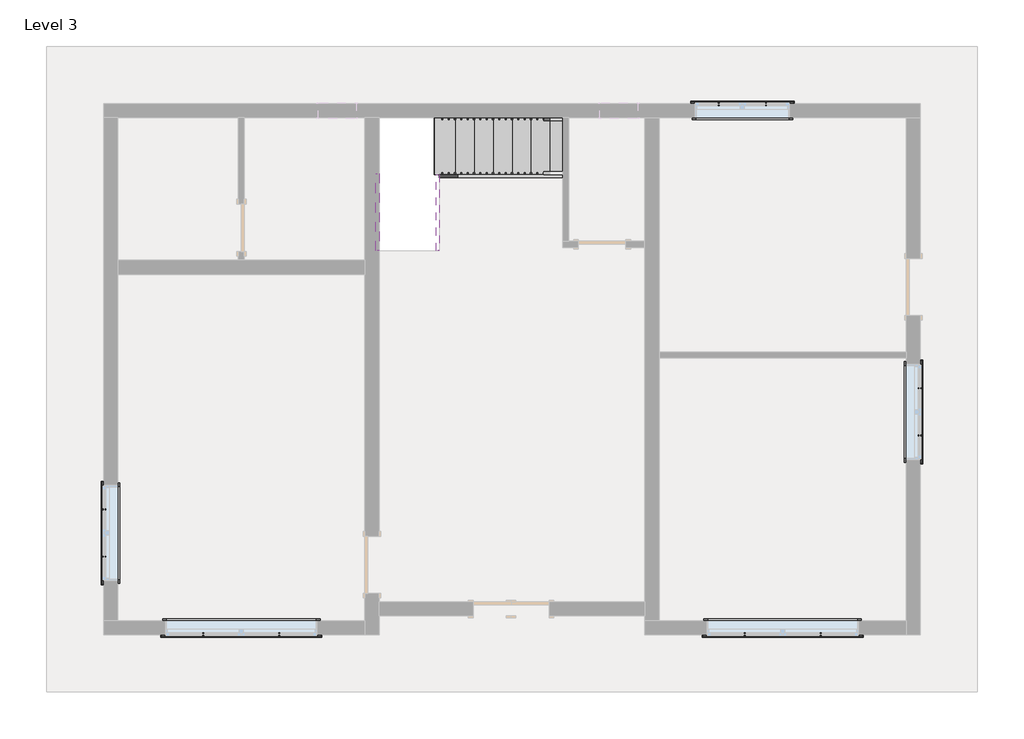
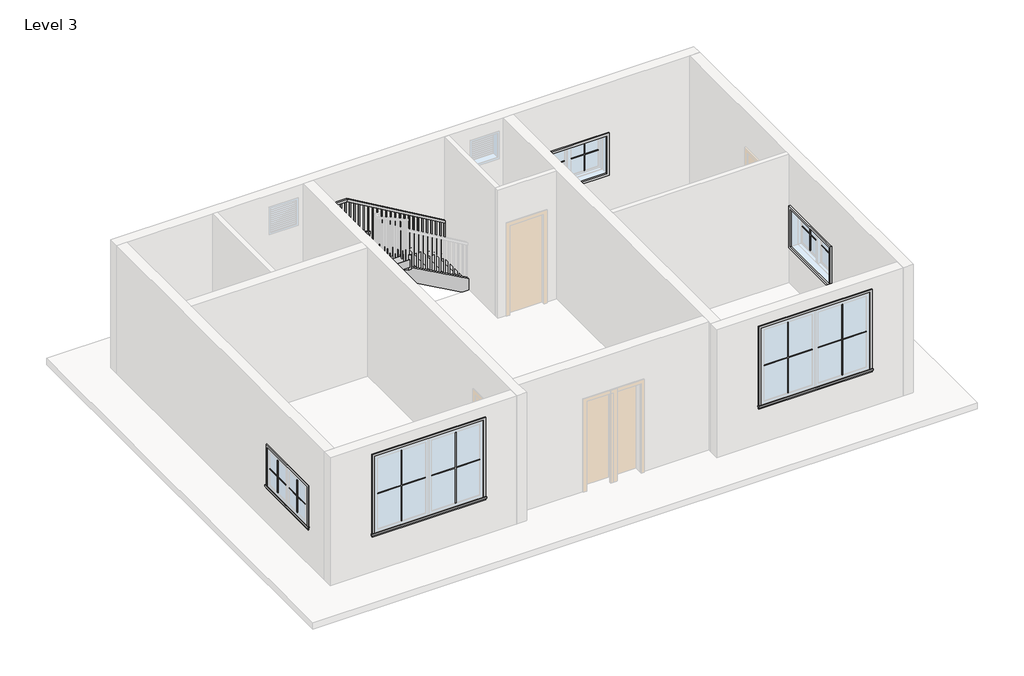
# One storey, part 2 of 2: 20 proxies, 4 members, 1 railing, 1 stair flight.
"""IFC4 building model written with IfcOpenShell, lengths in millimetres."""

from ifc_helpers import new_model, si_unit, frame, origin, place, context, project, spatial, polyline, outline, extrude, faceted_brep, transform, mapped, element, save
from components import muntin_pattern_2x2_muntin_pattern_2x2_9352d081, muntin_pattern_2x2_muntin_pattern_2x2_5c2cbe28, muntin_pattern_2x2_muntin_pattern_2x2_bb8d4d84, muntin_pattern_2x2_muntin_pattern_2x2_d03a1f3c, trim_window_exterior_flat_with_sill_979bde60, trim_window_exterior_flat_with_sill_359ed2ce, trim_window_interior_flat_picture_frame_7883d11b, trim_window_interior_flat_picture_frame_939a8053, stair_flight_1226b75b

model = new_model("IFC4")

# Units and contexts
model_context = context("Model", 3, world=origin())
ifc_project = project(units=[si_unit("LENGTHUNIT", "METRE", prefix="MILLI")], contexts=[model_context])

# Site, building, storey
site = spatial("IfcSite", under=ifc_project)
building = spatial("IfcBuilding", under=site)
storey = spatial("IfcBuildingStorey", under=building, Name="Level 3", Elevation=6248.4)

# Proxies
placement = place(None, origin())
muntin_pattern_2x2_muntin_pattern_2x2_shape = muntin_pattern_2x2_muntin_pattern_2x2_9352d081(model_context)
element("IfcBuildingElementProxy", 1, Name="Muntin Pattern_2x2 : Muntin Pattern_2x2", ObjectType="Muntin Pattern_2x2 : Muntin Pattern_2x2", at=placement, inside=storey, context=model_context, shape_type="MappedRepresentation", body=[
    mapped(muntin_pattern_2x2_muntin_pattern_2x2_shape, transform((-7798.9165084, -1764.5743005, 7232.65), x_axis=(0.0, 1.0, 0.0), y_axis=(-1.0, 0.0, 0.0), z_axis=(0.0, 0.0, 1.0))),
])
element("IfcBuildingElementProxy", 2, Name="Muntin Pattern_2x2 : Muntin Pattern_2x2", ObjectType="Muntin Pattern_2x2 : Muntin Pattern_2x2", at=placement, inside=storey, context=model_context, shape_type="MappedRepresentation", body=[
    mapped(muntin_pattern_2x2_muntin_pattern_2x2_shape, transform((5288.4334916, 937.3506995, 7232.65), x_axis=(0.0, -1.0, 0.0), y_axis=(1.0, 0.0, 0.0), z_axis=(0.0, 0.0, 1.0))),
])
element("IfcBuildingElementProxy", 3, Name="Muntin Pattern_2x2 : Muntin Pattern_2x2", ObjectType="Muntin Pattern_2x2 : Muntin Pattern_2x2", at=placement, inside=storey, context=model_context, shape_type="MappedRepresentation", body=[
    mapped(muntin_pattern_2x2_muntin_pattern_2x2_shape, transform((2061.0459916, 5501.4131995, 7232.65), x_axis=(1.0, 0.0, 0.0), y_axis=(0.0, 1.0, 0.0), z_axis=(0.0, 0.0, 1.0))),
])
muntin_pattern_2x2_muntin_pattern_2x2_2_shape = muntin_pattern_2x2_muntin_pattern_2x2_5c2cbe28(model_context)
element("IfcBuildingElementProxy", 4, Name="Muntin Pattern_2x2 : Muntin Pattern_2x2", ObjectType="Muntin Pattern_2x2 : Muntin Pattern_2x2", at=placement, inside=storey, context=model_context, shape_type="MappedRepresentation", body=[
    mapped(muntin_pattern_2x2_muntin_pattern_2x2_2_shape, transform((-7798.9165084, -1005.7493005, 7232.65), x_axis=(0.0, -1.0, 0.0), y_axis=(1.0, 0.0, 0.0), z_axis=(0.0, 0.0, 1.0))),
])
element("IfcBuildingElementProxy", 5, Name="Muntin Pattern_2x2 : Muntin Pattern_2x2", ObjectType="Muntin Pattern_2x2 : Muntin Pattern_2x2", at=placement, inside=storey, context=model_context, shape_type="MappedRepresentation", body=[
    mapped(muntin_pattern_2x2_muntin_pattern_2x2_2_shape, transform((5288.4334916, 178.5256995, 7232.65), x_axis=(0.0, 1.0, 0.0), y_axis=(-1.0, 0.0, 0.0), z_axis=(0.0, 0.0, 1.0))),
])
element("IfcBuildingElementProxy", 6, Name="Muntin Pattern_2x2 : Muntin Pattern_2x2", ObjectType="Muntin Pattern_2x2 : Muntin Pattern_2x2", at=placement, inside=storey, context=model_context, shape_type="MappedRepresentation", body=[
    mapped(muntin_pattern_2x2_muntin_pattern_2x2_2_shape, transform((2819.8709916, 5501.4131995, 7232.65), x_axis=(-1.0, 0.0, 0.0), y_axis=(0.0, -1.0, 0.0), z_axis=(0.0, 0.0, 1.0))),
])
muntin_pattern_2x2_muntin_pattern_2x2_3_shape = muntin_pattern_2x2_muntin_pattern_2x2_bb8d4d84(model_context)
element("IfcBuildingElementProxy", 7, Name="Muntin Pattern_2x2 : Muntin Pattern_2x2", ObjectType="Muntin Pattern_2x2 : Muntin Pattern_2x2", at=placement, inside=storey, context=model_context, shape_type="MappedRepresentation", body=[
    mapped(muntin_pattern_2x2_muntin_pattern_2x2_3_shape, transform((-4990.6290084, -3013.9368005, 7232.65), x_axis=(-1.0, 0.0, 0.0), y_axis=(0.0, -1.0, 0.0), z_axis=(0.0, 0.0, 1.0))),
])
element("IfcBuildingElementProxy", 8, Name="Muntin Pattern_2x2 : Muntin Pattern_2x2", ObjectType="Muntin Pattern_2x2 : Muntin Pattern_2x2", at=placement, inside=storey, context=model_context, shape_type="MappedRepresentation", body=[
    mapped(muntin_pattern_2x2_muntin_pattern_2x2_3_shape, transform((3696.1709916, -3013.9368005, 7232.65), x_axis=(-1.0, 0.0, 0.0), y_axis=(0.0, -1.0, 0.0), z_axis=(0.0, 0.0, 1.0))),
])
muntin_pattern_2x2_muntin_pattern_2x2_4_shape = muntin_pattern_2x2_muntin_pattern_2x2_d03a1f3c(model_context)
element("IfcBuildingElementProxy", 9, Name="Muntin Pattern_2x2 : Muntin Pattern_2x2", ObjectType="Muntin Pattern_2x2 : Muntin Pattern_2x2", at=placement, inside=storey, context=model_context, shape_type="MappedRepresentation", body=[
    mapped(muntin_pattern_2x2_muntin_pattern_2x2_4_shape, transform((-6206.6540084, -3013.9368005, 7232.65), x_axis=(1.0, 0.0, 0.0), y_axis=(0.0, 1.0, 0.0), z_axis=(0.0, 0.0, 1.0))),
])
element("IfcBuildingElementProxy", 10, Name="Muntin Pattern_2x2 : Muntin Pattern_2x2", ObjectType="Muntin Pattern_2x2 : Muntin Pattern_2x2", at=placement, inside=storey, context=model_context, shape_type="MappedRepresentation", body=[
    mapped(muntin_pattern_2x2_muntin_pattern_2x2_4_shape, transform((2480.1459916, -3013.9368005, 7232.65), x_axis=(1.0, 0.0, 0.0), y_axis=(0.0, 1.0, 0.0), z_axis=(0.0, 0.0, 1.0))),
])
trim_window_exterior_flat_with_sill_shape = trim_window_exterior_flat_with_sill_979bde60(model_context)
element("IfcBuildingElementProxy", 11, Name="Trim-Window-Exterior-Flat : with Sill", ObjectType="Trim-Window-Exterior-Flat : with Sill", at=placement, inside=storey, context=model_context, shape_type="MappedRepresentation", body=[
    mapped(trim_window_exterior_flat_with_sill_shape, transform((-7808.4415084, -1385.1618005, 8077.2), x_axis=(0.0, -1.0, 0.0), y_axis=(0.0, 0.0, 1.0), z_axis=(-1.0, 0.0, 0.0))),
])
element("IfcBuildingElementProxy", 12, Name="Trim-Window-Exterior-Flat : with Sill", ObjectType="Trim-Window-Exterior-Flat : with Sill", at=placement, inside=storey, context=model_context, shape_type="MappedRepresentation", body=[
    mapped(trim_window_exterior_flat_with_sill_shape, transform((5297.9584916, 557.9381995, 8077.2), x_axis=(0.0, 1.0, 0.0), y_axis=(0.0, 0.0, 1.0), z_axis=(1.0, 0.0, 0.0))),
])
element("IfcBuildingElementProxy", 13, Name="Trim-Window-Exterior-Flat : with Sill", ObjectType="Trim-Window-Exterior-Flat : with Sill", at=placement, inside=storey, context=model_context, shape_type="MappedRepresentation", body=[
    mapped(trim_window_exterior_flat_with_sill_shape, transform((2440.4584916, 5510.9381995, 8077.2), x_axis=(-1.0, 0.0, 0.0), y_axis=(0.0, 0.0, 1.0), z_axis=(0.0, 1.0, 0.0))),
])
trim_window_exterior_flat_with_sill_2_shape = trim_window_exterior_flat_with_sill_359ed2ce(model_context)
element("IfcBuildingElementProxy", 14, Name="Trim-Window-Exterior-Flat : with Sill", ObjectType="Trim-Window-Exterior-Flat : with Sill", at=placement, inside=storey, context=model_context, shape_type="MappedRepresentation", body=[
    mapped(trim_window_exterior_flat_with_sill_2_shape, transform((-5598.6415084, -3023.4618005, 8991.6), x_axis=(1.0, 0.0, 0.0), y_axis=(0.0, 0.0, 1.0), z_axis=(0.0, -1.0, 0.0))),
])
element("IfcBuildingElementProxy", 15, Name="Trim-Window-Exterior-Flat : with Sill", ObjectType="Trim-Window-Exterior-Flat : with Sill", at=placement, inside=storey, context=model_context, shape_type="MappedRepresentation", body=[
    mapped(trim_window_exterior_flat_with_sill_2_shape, transform((3088.1584916, -3023.4618005, 8991.6), x_axis=(1.0, 0.0, 0.0), y_axis=(0.0, 0.0, 1.0), z_axis=(0.0, -1.0, 0.0))),
])
trim_window_interior_flat_picture_frame_shape = trim_window_interior_flat_picture_frame_7883d11b(model_context)
element("IfcBuildingElementProxy", 16, Name="Trim-Window-Interior-Flat : Picture Frame", ObjectType="Trim-Window-Interior-Flat : Picture Frame", at=placement, inside=storey, context=model_context, shape_type="MappedRepresentation", body=[
    mapped(trim_window_interior_flat_picture_frame_shape, transform((-7579.8415084, -1385.1618005, 8077.2), x_axis=(0.0, 1.0, 0.0), y_axis=(0.0, 0.0, 1.0), z_axis=(1.0, 0.0, 0.0))),
])
element("IfcBuildingElementProxy", 17, Name="Trim-Window-Interior-Flat : Picture Frame", ObjectType="Trim-Window-Interior-Flat : Picture Frame", at=placement, inside=storey, context=model_context, shape_type="MappedRepresentation", body=[
    mapped(trim_window_interior_flat_picture_frame_shape, transform((5069.3584916, 557.9381995, 8077.2), x_axis=(0.0, -1.0, 0.0), y_axis=(0.0, 0.0, 1.0), z_axis=(-1.0, 0.0, 0.0))),
])
element("IfcBuildingElementProxy", 18, Name="Trim-Window-Interior-Flat : Picture Frame", ObjectType="Trim-Window-Interior-Flat : Picture Frame", at=placement, inside=storey, context=model_context, shape_type="MappedRepresentation", body=[
    mapped(trim_window_interior_flat_picture_frame_shape, transform((2440.4584916, 5282.3381995, 8077.2), x_axis=(1.0, 0.0, 0.0), y_axis=(0.0, 0.0, 1.0), z_axis=(0.0, -1.0, 0.0))),
])
trim_window_interior_flat_picture_frame_2_shape = trim_window_interior_flat_picture_frame_939a8053(model_context)
element("IfcBuildingElementProxy", 19, Name="Trim-Window-Interior-Flat : Picture Frame", ObjectType="Trim-Window-Interior-Flat : Picture Frame", at=placement, inside=storey, context=model_context, shape_type="MappedRepresentation", body=[
    mapped(trim_window_interior_flat_picture_frame_2_shape, transform((-5598.6415084, -2794.8618005, 8991.6), x_axis=(-1.0, 0.0, 0.0), y_axis=(0.0, 0.0, 1.0), z_axis=(0.0, 1.0, 0.0))),
])
element("IfcBuildingElementProxy", 20, Name="Trim-Window-Interior-Flat : Picture Frame", ObjectType="Trim-Window-Interior-Flat : Picture Frame", at=placement, inside=storey, context=model_context, shape_type="MappedRepresentation", body=[
    mapped(trim_window_interior_flat_picture_frame_2_shape, transform((3088.1584916, -2794.8618005, 8991.6), x_axis=(-1.0, 0.0, 0.0), y_axis=(0.0, 0.0, 1.0), z_axis=(0.0, 1.0, 0.0))),
])

# Members
element("IfcMember", 21, ObjectType="Stringer - 2\" Width", at=placement, inside=storey, context=model_context, shape_type="SweptSolid", body=[
    extrude(outline(polyline([(6248.4, -442.4415084), (6512.4428392, -442.4415084), (7613.1095059, -2423.6415084), (7264.4308318, -2423.6415084), (6248.4, -594.7860112), (6248.4, -442.4415084)])), frame((0.0, 4317.5146777, 0.0), z_axis=(0.0, 1.0, 0.0), x_axis=(0.0, 0.0, 1.0)), (0.0, 0.0, 1.0), 50.8),
])
element("IfcMember", 22, ObjectType="Stringer - 2\" Width", at=placement, inside=storey, context=model_context, shape_type="SweptSolid", body=[
    extrude(outline(polyline([(4368.3146777, 7810.645537), (4368.3146777, 7462.0006925), (3148.7383287, 8139.2643411), (3148.7383287, 8487.9091856), (4368.3146777, 7810.645537)])), frame((-2474.4415084, 0.0, 0.0), z_axis=(1.0, 0.0, 0.0), x_axis=(0.0, 1.0, 0.0)), (0.0, 0.0, 1.0), 50.8),
])
element("IfcMember", 23, ObjectType="Stringer - 2\" Width", at=placement, inside=storey, context=model_context, shape_type="SweptSolid", body=[
    extrude(outline(polyline([(6248.4, -442.4415084), (6512.4428392, -442.4415084), (7303.0636166, -1865.5589077), (7303.0636166, -2493.1805211), (6248.4, -594.7860112), (6248.4, -442.4415084)])), frame((0.0, 5282.3381995, 0.0), z_axis=(0.0, 1.0, 0.0), x_axis=(0.0, 0.0, 1.0)), (0.0, 0.0, 1.0), 50.8),
])
element("IfcMember", 24, ObjectType="Stringer - 2\" Width", at=placement, inside=storey, context=model_context, shape_type="SweptSolid", body=[
    extrude(outline(polyline([(3758.489521, 7800.653054), (3148.7383287, 8139.2643411), (3148.7383287, 8487.9091856), (4386.3085505, 7800.653054), (3758.489521, 7800.653054)])), frame((-3439.6415084, 0.0, 0.0), z_axis=(1.0, 0.0, 0.0), x_axis=(0.0, 1.0, 0.0)), (0.0, 0.0, 1.0), 50.8),
])

# Railing
element("IfcRailing", 25, ObjectType="Handrail - Rectangular", at=placement, inside=storey, context=model_context, shape_type="SolidModel", body=[
    faceted_brep([(-442.4415084, 5231.5381995, 7332.1333333), (-442.4415084, 5231.5381995, 7273.3219871), (-442.4415084, 5282.3381995, 7273.3219871), (-442.4415084, 5282.3381995, 7332.1333333), (-2641.0608886, 5231.5381995, 8614.6613051), (-2654.794625, 5231.5381995, 8563.8613051), (-2654.794625, 5282.3381995, 8563.8613051), (-2641.0608886, 5282.3381995, 8614.6613051), (-3338.0415084, 5231.5381995, 8614.6613051), (-3338.0415084, 5231.5381995, 8563.8613051), (-3388.8415084, 5282.3381995, 8563.8613051), (-3388.8415084, 5282.3381995, 8614.6613051), (-3338.0415084, 4498.2044111, 8614.6613051), (-3338.0415084, 4485.04436, 8563.8613051), (-3388.8415084, 4485.04436, 8563.8613051), (-3388.8415084, 4498.2044111, 8614.6613051), (-3338.0415084, 3148.7383287, 9364.1333333), (-3388.8415084, 3148.7383287, 9364.1333333), (-3388.8415084, 3148.7383287, 9306.02445), (-3338.0415084, 3148.7383287, 9306.02445)], [[[0, 1, 2, 3]], [[1, 0, 4, 5]], [[2, 1, 5, 6]], [[3, 2, 6, 7]], [[0, 3, 7, 4]], [[5, 4, 8, 9]], [[6, 5, 9, 10]], [[7, 6, 10, 11]], [[4, 7, 11, 8]], [[9, 8, 12, 13]], [[10, 9, 13, 14]], [[11, 10, 14, 15]], [[8, 11, 15, 12]], [[16, 17, 18, 19]], [[13, 12, 16, 19]], [[14, 13, 19, 18]], [[15, 14, 18, 17]], [[12, 15, 17, 16]]]),
    extrude(outline(polyline([(3215.4131995, 9268.9942858), (3234.4631995, 9258.4142183), (3234.4631995, 8280.4), (3215.4131995, 8280.4), (3215.4131995, 9268.9942858)])), frame((-3372.9665084, 0.0, 0.0), z_axis=(1.0, 0.0, 0.0), x_axis=(0.0, 1.0, 0.0)), (0.0, 0.0, 1.0), 19.05),
    extrude(outline(polyline([(3317.0131995, 9212.7240232), (3336.0631995, 9202.1439558), (3336.0631995, 8280.4), (3317.0131995, 8280.4), (3317.0131995, 9212.7240232)])), frame((-3372.9665084, 0.0, 0.0), z_axis=(1.0, 0.0, 0.0), x_axis=(0.0, 1.0, 0.0)), (0.0, 0.0, 1.0), 19.05),
    extrude(outline(polyline([(3418.6131995, 9156.2969969), (3437.6631995, 9145.7169295), (3437.6631995, 8280.4), (3418.6131995, 8280.4), (3418.6131995, 9156.2969969)])), frame((-3372.9665084, 0.0, 0.0), z_axis=(1.0, 0.0, 0.0), x_axis=(0.0, 1.0, 0.0)), (0.0, 0.0, 1.0), 19.05),
    extrude(outline(polyline([(3520.2131995, 9099.8699707), (3539.2631995, 9089.2899033), (3539.2631995, 8111.0666667), (3520.2131995, 8111.0666667), (3520.2131995, 9099.8699707)])), frame((-3372.9665084, 0.0, 0.0), z_axis=(1.0, 0.0, 0.0), x_axis=(0.0, 1.0, 0.0)), (0.0, 0.0, 1.0), 19.05),
    extrude(outline(polyline([(3621.8131995, 9043.3906899), (3640.8631995, 9032.8106224), (3640.8631995, 8111.0666667), (3621.8131995, 8111.0666667), (3621.8131995, 9043.3906899)])), frame((-3372.9665084, 0.0, 0.0), z_axis=(1.0, 0.0, 0.0), x_axis=(0.0, 1.0, 0.0)), (0.0, 0.0, 1.0), 19.05),
    extrude(outline(polyline([(3723.4131995, 8986.9636636), (3742.4631995, 8976.3835962), (3742.4631995, 8111.0666667), (3723.4131995, 8111.0666667), (3723.4131995, 8986.9636636)])), frame((-3372.9665084, 0.0, 0.0), z_axis=(1.0, 0.0, 0.0), x_axis=(0.0, 1.0, 0.0)), (0.0, 0.0, 1.0), 19.05),
    extrude(outline(polyline([(3825.0131995, 8930.5366374), (3844.0631995, 8919.9565699), (3844.0631995, 7941.7333333), (3825.0131995, 7941.7333333), (3825.0131995, 8930.5366374)])), frame((-3372.9665084, 0.0, 0.0), z_axis=(1.0, 0.0, 0.0), x_axis=(0.0, 1.0, 0.0)), (0.0, 0.0, 1.0), 19.05),
    extrude(outline(polyline([(3926.6131995, 8874.0573565), (3945.6631995, 8863.4772891), (3945.6631995, 7941.7333333), (3926.6131995, 7941.7333333), (3926.6131995, 8874.0573565)])), frame((-3372.9665084, 0.0, 0.0), z_axis=(1.0, 0.0, 0.0), x_axis=(0.0, 1.0, 0.0)), (0.0, 0.0, 1.0), 19.05),
    extrude(outline(polyline([(4028.2131995, 8817.6303303), (4047.2631995, 8807.0502629), (4047.2631995, 7941.7333333), (4028.2131995, 7941.7333333), (4028.2131995, 8817.6303303)])), frame((-3372.9665084, 0.0, 0.0), z_axis=(1.0, 0.0, 0.0), x_axis=(0.0, 1.0, 0.0)), (0.0, 0.0, 1.0), 19.05),
    extrude(outline(polyline([(4129.8131995, 8761.203304), (4148.8631995, 8750.6232366), (4148.8631995, 7772.4), (4129.8131995, 7772.4), (4129.8131995, 8761.203304)])), frame((-3372.9665084, 0.0, 0.0), z_axis=(1.0, 0.0, 0.0), x_axis=(0.0, 1.0, 0.0)), (0.0, 0.0, 1.0), 19.05),
    extrude(outline(polyline([(4231.4131995, 8704.7240232), (4250.4631995, 8694.1439558), (4250.4631995, 7772.4), (4231.4131995, 7772.4), (4231.4131995, 8704.7240232)])), frame((-3372.9665084, 0.0, 0.0), z_axis=(1.0, 0.0, 0.0), x_axis=(0.0, 1.0, 0.0)), (0.0, 0.0, 1.0), 19.05),
    extrude(outline(polyline([(4333.0131995, 8648.2969969), (4352.0631995, 8637.7169295), (4352.0631995, 7772.4), (4333.0131995, 7772.4), (4333.0131995, 8648.2969969)])), frame((-3372.9665084, 0.0, 0.0), z_axis=(1.0, 0.0, 0.0), x_axis=(0.0, 1.0, 0.0)), (0.0, 0.0, 1.0), 19.05),
    extrude(outline(polyline([(4434.6131995, 8591.8699707), (4453.6631995, 8581.2899033), (4453.6631995, 7603.0666667), (4434.6131995, 7603.0666667), (4434.6131995, 8591.8699707)])), frame((-3372.9665084, 0.0, 0.0), z_axis=(1.0, 0.0, 0.0), x_axis=(0.0, 1.0, 0.0)), (0.0, 0.0, 1.0), 19.05),
    extrude(outline(polyline([(-3372.9665084, 4555.2631995), (-3353.9165084, 4555.2631995), (-3353.9165084, 4536.2131995), (-3372.9665084, 4536.2131995), (-3372.9665084, 4555.2631995)])), frame((0.0, 0.0, 7603.0666667), z_axis=(0.0, 0.0, 1.0), x_axis=(1.0, 0.0, 0.0)), (0.0, 0.0, 1.0), 960.7946385),
    extrude(outline(polyline([(-3372.9665084, 4656.8631995), (-3353.9165084, 4656.8631995), (-3353.9165084, 4637.8131995), (-3372.9665084, 4637.8131995), (-3372.9665084, 4656.8631995)])), frame((0.0, 0.0, 7603.0666667), z_axis=(0.0, 0.0, 1.0), x_axis=(1.0, 0.0, 0.0)), (0.0, 0.0, 1.0), 960.7946385),
    extrude(outline(polyline([(-3372.9665084, 4758.4631995), (-3353.9165084, 4758.4631995), (-3353.9165084, 4739.4131995), (-3372.9665084, 4739.4131995), (-3372.9665084, 4758.4631995)])), frame((0.0, 0.0, 7603.0666667), z_axis=(0.0, 0.0, 1.0), x_axis=(1.0, 0.0, 0.0)), (0.0, 0.0, 1.0), 960.7946385),
    extrude(outline(polyline([(-3372.9665084, 4860.0631995), (-3353.9165084, 4860.0631995), (-3353.9165084, 4841.0131995), (-3372.9665084, 4841.0131995), (-3372.9665084, 4860.0631995)])), frame((0.0, 0.0, 7603.0666667), z_axis=(0.0, 0.0, 1.0), x_axis=(1.0, 0.0, 0.0)), (0.0, 0.0, 1.0), 960.7946385),
    extrude(outline(polyline([(-3372.9665084, 4961.6631995), (-3353.9165084, 4961.6631995), (-3353.9165084, 4942.6131995), (-3372.9665084, 4942.6131995), (-3372.9665084, 4961.6631995)])), frame((0.0, 0.0, 7603.0666667), z_axis=(0.0, 0.0, 1.0), x_axis=(1.0, 0.0, 0.0)), (0.0, 0.0, 1.0), 960.7946385),
    extrude(outline(polyline([(-3372.9665084, 5063.2631995), (-3353.9165084, 5063.2631995), (-3353.9165084, 5044.2131995), (-3372.9665084, 5044.2131995), (-3372.9665084, 5063.2631995)])), frame((0.0, 0.0, 7603.0666667), z_axis=(0.0, 0.0, 1.0), x_axis=(1.0, 0.0, 0.0)), (0.0, 0.0, 1.0), 960.7946385),
    extrude(outline(polyline([(-3372.9665084, 5164.8631995), (-3353.9165084, 5164.8631995), (-3353.9165084, 5145.8131995), (-3372.9665084, 5145.8131995), (-3372.9665084, 5164.8631995)])), frame((0.0, 0.0, 7603.0666667), z_axis=(0.0, 0.0, 1.0), x_axis=(1.0, 0.0, 0.0)), (0.0, 0.0, 1.0), 960.7946385),
    extrude(outline(polyline([(-3277.7165084, 5266.4631995), (-3277.7165084, 5247.4131995), (-3296.7665084, 5247.4131995), (-3296.7665084, 5266.4631995), (-3277.7165084, 5266.4631995)])), frame((0.0, 0.0, 7603.0666667), z_axis=(0.0, 0.0, 1.0), x_axis=(1.0, 0.0, 0.0)), (0.0, 0.0, 1.0), 960.7946385),
    extrude(outline(polyline([(-3176.1165084, 5266.4631995), (-3176.1165084, 5247.4131995), (-3195.1665084, 5247.4131995), (-3195.1665084, 5266.4631995), (-3176.1165084, 5266.4631995)])), frame((0.0, 0.0, 7603.0666667), z_axis=(0.0, 0.0, 1.0), x_axis=(1.0, 0.0, 0.0)), (0.0, 0.0, 1.0), 960.7946385),
    extrude(outline(polyline([(-3074.5165084, 5266.4631995), (-3074.5165084, 5247.4131995), (-3093.5665084, 5247.4131995), (-3093.5665084, 5266.4631995), (-3074.5165084, 5266.4631995)])), frame((0.0, 0.0, 7603.0666667), z_axis=(0.0, 0.0, 1.0), x_axis=(1.0, 0.0, 0.0)), (0.0, 0.0, 1.0), 960.7946385),
    extrude(outline(polyline([(-2972.9165084, 5266.4631995), (-2972.9165084, 5247.4131995), (-2991.9665084, 5247.4131995), (-2991.9665084, 5266.4631995), (-2972.9165084, 5266.4631995)])), frame((0.0, 0.0, 7603.0666667), z_axis=(0.0, 0.0, 1.0), x_axis=(1.0, 0.0, 0.0)), (0.0, 0.0, 1.0), 960.7946385),
    extrude(outline(polyline([(-2871.3165084, 5266.4631995), (-2871.3165084, 5247.4131995), (-2890.3665084, 5247.4131995), (-2890.3665084, 5266.4631995), (-2871.3165084, 5266.4631995)])), frame((0.0, 0.0, 7603.0666667), z_axis=(0.0, 0.0, 1.0), x_axis=(1.0, 0.0, 0.0)), (0.0, 0.0, 1.0), 960.7946385),
    extrude(outline(polyline([(-2769.7165084, 5266.4631995), (-2769.7165084, 5247.4131995), (-2788.7665084, 5247.4131995), (-2788.7665084, 5266.4631995), (-2769.7165084, 5266.4631995)])), frame((0.0, 0.0, 7603.0666667), z_axis=(0.0, 0.0, 1.0), x_axis=(1.0, 0.0, 0.0)), (0.0, 0.0, 1.0), 960.7946385),
    extrude(outline(polyline([(-2668.1165084, 5266.4631995), (-2668.1165084, 5247.4131995), (-2687.1665084, 5247.4131995), (-2687.1665084, 5266.4631995), (-2668.1165084, 5266.4631995)])), frame((0.0, 0.0, 7603.0666667), z_axis=(0.0, 0.0, 1.0), x_axis=(1.0, 0.0, 0.0)), (0.0, 0.0, 1.0), 960.7946385),
    extrude(outline(polyline([(8512.3657371, -2566.5165084), (8523.4782371, -2585.5665084), (7603.0666667, -2585.5665084), (7603.0666667, -2566.5165084), (8512.3657371, -2566.5165084)])), frame((0.0, 5247.4131995, 0.0), z_axis=(0.0, 1.0, 0.0), x_axis=(0.0, 0.0, 1.0)), (0.0, 0.0, 1.0), 19.05),
    extrude(outline(polyline([(8453.0990704, -2464.9165084), (8464.2115704, -2483.9665084), (7603.0666667, -2483.9665084), (7603.0666667, -2464.9165084), (8453.0990704, -2464.9165084)])), frame((0.0, 5247.4131995, 0.0), z_axis=(0.0, 1.0, 0.0), x_axis=(0.0, 0.0, 1.0)), (0.0, 0.0, 1.0), 19.05),
    extrude(outline(polyline([(8393.8324038, -2363.3165084), (8404.9449038, -2382.3665084), (7433.7333333, -2382.3665084), (7433.7333333, -2363.3165084), (8393.8324038, -2363.3165084)])), frame((0.0, 5247.4131995, 0.0), z_axis=(0.0, 1.0, 0.0), x_axis=(0.0, 0.0, 1.0)), (0.0, 0.0, 1.0), 19.05),
    extrude(outline(polyline([(8334.5657371, -2261.7165084), (8345.6782371, -2280.7665084), (7433.7333333, -2280.7665084), (7433.7333333, -2261.7165084), (8334.5657371, -2261.7165084)])), frame((0.0, 5247.4131995, 0.0), z_axis=(0.0, 1.0, 0.0), x_axis=(0.0, 0.0, 1.0)), (0.0, 0.0, 1.0), 19.05),
    extrude(outline(polyline([(8275.2990704, -2160.1165084), (8286.4115704, -2179.1665084), (7433.7333333, -2179.1665084), (7433.7333333, -2160.1165084), (8275.2990704, -2160.1165084)])), frame((0.0, 5247.4131995, 0.0), z_axis=(0.0, 1.0, 0.0), x_axis=(0.0, 0.0, 1.0)), (0.0, 0.0, 1.0), 19.05),
    extrude(outline(polyline([(8216.0324038, -2058.5165084), (8227.1449038, -2077.5665084), (7264.4, -2077.5665084), (7264.4, -2058.5165084), (8216.0324038, -2058.5165084)])), frame((0.0, 5247.4131995, 0.0), z_axis=(0.0, 1.0, 0.0), x_axis=(0.0, 0.0, 1.0)), (0.0, 0.0, 1.0), 19.05),
    extrude(outline(polyline([(8156.7657371, -1956.9165084), (8167.8782371, -1975.9665084), (7264.4, -1975.9665084), (7264.4, -1956.9165084), (8156.7657371, -1956.9165084)])), frame((0.0, 5247.4131995, 0.0), z_axis=(0.0, 1.0, 0.0), x_axis=(0.0, 0.0, 1.0)), (0.0, 0.0, 1.0), 19.05),
    extrude(outline(polyline([(8097.4990704, -1855.3165084), (8108.6115704, -1874.3665084), (7264.4, -1874.3665084), (7264.4, -1855.3165084), (8097.4990704, -1855.3165084)])), frame((0.0, 5247.4131995, 0.0), z_axis=(0.0, 1.0, 0.0), x_axis=(0.0, 0.0, 1.0)), (0.0, 0.0, 1.0), 19.05),
    extrude(outline(polyline([(8038.2324038, -1753.7165084), (8049.3449038, -1772.7665084), (7095.0666667, -1772.7665084), (7095.0666667, -1753.7165084), (8038.2324038, -1753.7165084)])), frame((0.0, 5247.4131995, 0.0), z_axis=(0.0, 1.0, 0.0), x_axis=(0.0, 0.0, 1.0)), (0.0, 0.0, 1.0), 19.05),
    extrude(outline(polyline([(7978.9657371, -1652.1165084), (7990.0782371, -1671.1665084), (7095.0666667, -1671.1665084), (7095.0666667, -1652.1165084), (7978.9657371, -1652.1165084)])), frame((0.0, 5247.4131995, 0.0), z_axis=(0.0, 1.0, 0.0), x_axis=(0.0, 0.0, 1.0)), (0.0, 0.0, 1.0), 19.05),
    extrude(outline(polyline([(7919.6990704, -1550.5165084), (7930.8115704, -1569.5665084), (7095.0666667, -1569.5665084), (7095.0666667, -1550.5165084), (7919.6990704, -1550.5165084)])), frame((0.0, 5247.4131995, 0.0), z_axis=(0.0, 1.0, 0.0), x_axis=(0.0, 0.0, 1.0)), (0.0, 0.0, 1.0), 19.05),
    extrude(outline(polyline([(7860.4324038, -1448.9165084), (7871.5449038, -1467.9665084), (6925.7333333, -1467.9665084), (6925.7333333, -1448.9165084), (7860.4324038, -1448.9165084)])), frame((0.0, 5247.4131995, 0.0), z_axis=(0.0, 1.0, 0.0), x_axis=(0.0, 0.0, 1.0)), (0.0, 0.0, 1.0), 19.05),
    extrude(outline(polyline([(7801.1657371, -1347.3165084), (7812.2782371, -1366.3665084), (6925.7333333, -1366.3665084), (6925.7333333, -1347.3165084), (7801.1657371, -1347.3165084)])), frame((0.0, 5247.4131995, 0.0), z_axis=(0.0, 1.0, 0.0), x_axis=(0.0, 0.0, 1.0)), (0.0, 0.0, 1.0), 19.05),
    extrude(outline(polyline([(7741.8990704, -1245.7165084), (7753.0115704, -1264.7665084), (6925.7333333, -1264.7665084), (6925.7333333, -1245.7165084), (7741.8990704, -1245.7165084)])), frame((0.0, 5247.4131995, 0.0), z_axis=(0.0, 1.0, 0.0), x_axis=(0.0, 0.0, 1.0)), (0.0, 0.0, 1.0), 19.05),
    extrude(outline(polyline([(7682.6324038, -1144.1165084), (7693.7449038, -1163.1665084), (6756.4, -1163.1665084), (6756.4, -1144.1165084), (7682.6324038, -1144.1165084)])), frame((0.0, 5247.4131995, 0.0), z_axis=(0.0, 1.0, 0.0), x_axis=(0.0, 0.0, 1.0)), (0.0, 0.0, 1.0), 19.05),
    extrude(outline(polyline([(7623.3657371, -1042.5165084), (7634.4782371, -1061.5665084), (6756.4, -1061.5665084), (6756.4, -1042.5165084), (7623.3657371, -1042.5165084)])), frame((0.0, 5247.4131995, 0.0), z_axis=(0.0, 1.0, 0.0), x_axis=(0.0, 0.0, 1.0)), (0.0, 0.0, 1.0), 19.05),
    extrude(outline(polyline([(7564.0990704, -940.9165084), (7575.2115704, -959.9665084), (6756.4, -959.9665084), (6756.4, -940.9165084), (7564.0990704, -940.9165084)])), frame((0.0, 5247.4131995, 0.0), z_axis=(0.0, 1.0, 0.0), x_axis=(0.0, 0.0, 1.0)), (0.0, 0.0, 1.0), 19.05),
    extrude(outline(polyline([(7504.8324038, -839.3165084), (7515.9449038, -858.3665084), (6587.0666667, -858.3665084), (6587.0666667, -839.3165084), (7504.8324038, -839.3165084)])), frame((0.0, 5247.4131995, 0.0), z_axis=(0.0, 1.0, 0.0), x_axis=(0.0, 0.0, 1.0)), (0.0, 0.0, 1.0), 19.05),
    extrude(outline(polyline([(7445.5657371, -737.7165084), (7456.6782371, -756.7665084), (6587.0666667, -756.7665084), (6587.0666667, -737.7165084), (7445.5657371, -737.7165084)])), frame((0.0, 5247.4131995, 0.0), z_axis=(0.0, 1.0, 0.0), x_axis=(0.0, 0.0, 1.0)), (0.0, 0.0, 1.0), 19.05),
    extrude(outline(polyline([(7386.2990704, -636.1165084), (7397.4115704, -655.1665084), (6587.0666667, -655.1665084), (6587.0666667, -636.1165084), (7386.2990704, -636.1165084)])), frame((0.0, 5247.4131995, 0.0), z_axis=(0.0, 1.0, 0.0), x_axis=(0.0, 0.0, 1.0)), (0.0, 0.0, 1.0), 19.05),
    extrude(outline(polyline([(7327.0324038, -534.5165084), (7338.1449038, -553.5665084), (6417.7333333, -553.5665084), (6417.7333333, -534.5165084), (7327.0324038, -534.5165084)])), frame((0.0, 5247.4131995, 0.0), z_axis=(0.0, 1.0, 0.0), x_axis=(0.0, 0.0, 1.0)), (0.0, 0.0, 1.0), 19.05),
    extrude(outline(polyline([(-3353.9165084, 5266.4631995), (-3353.9165084, 5247.4131995), (-3372.9665084, 5247.4131995), (-3372.9665084, 5266.4631995), (-3353.9165084, 5266.4631995)])), frame((0.0, 0.0, 7603.0666667), z_axis=(0.0, 0.0, 1.0), x_axis=(1.0, 0.0, 0.0)), (0.0, 0.0, 1.0), 960.7946385),
    extrude(outline(polyline([(3148.7383287, 9306.02445), (3167.7883287, 9295.4443826), (3167.7883287, 8280.4), (3148.7383287, 8280.4), (3148.7383287, 9306.02445)])), frame((-3372.9665084, 0.0, 0.0), z_axis=(1.0, 0.0, 0.0), x_axis=(0.0, 1.0, 0.0)), (0.0, 0.0, 1.0), 19.05),
    extrude(outline(polyline([(7273.3219871, -442.4415084), (7284.4344871, -461.4915084), (6417.7333333, -461.4915084), (6417.7333333, -442.4415084), (7273.3219871, -442.4415084)])), frame((0.0, 5247.4131995, 0.0), z_axis=(0.0, 1.0, 0.0), x_axis=(0.0, 0.0, 1.0)), (0.0, 0.0, 1.0), 19.05),
])

# Stair flight
stair_flight_shape = stair_flight_1226b75b(model_context)
element("IfcStairFlight", 26, ObjectType="2\" Tread 1\" Nosing 1/4\" Riser", at=placement, inside=storey, context=model_context, shape_type="MappedRepresentation", body=[
    mapped(stair_flight_shape, transform((0.0, 0.0, 0.0), x_axis=(1.0, 0.0, 0.0), y_axis=(0.0, 1.0, 0.0), z_axis=(0.0, 0.0, 1.0))),
])

save(model, "model.ifc")

# Revit data of these elements
# Type "Muntin Pattern_2x2 : Muntin Pattern_2x2"
#   Width [instance default] = 4' - 0"
#   Thickness = 0' - 0 1/2"
#   Height [instance default] = 4' - 0"
#   Distance = 0' - 0 3/4"
#   Interior Material [instance default] = none
#   Exterior Material [instance default] = none
#   Default Elevation = 0
# Type "Trim-Window-Exterior-Flat : with Sill"
#   Trim Width = 0' - 2 1/4"
#   Trim Thickness_Picture Frame = 0' - 1 1/4"
#   Trim Thickness_with Sill = 0' - 0 3/4"
#   Sill Thickness = 0' - 1 1/4"
#   Opening Width [instance default] = 2' - 0"
#   Opening Height [instance default] = 3' - 0"
#   Default Elevation = 4' - 0"
#   Sill = yes
#   Picture Frame = no
#   Trim Material [instance default] = none
# Type "Trim-Window-Interior-Flat : Picture Frame"
#   Trim Thickness_Picture Frame = 0' - 1 1/4"
#   Trim Width = 0' - 2 1/4"
#   Trim Thickness_with Sill = 0' - 0 3/4"
#   Sill Thickness = 0' - 1 1/4"
#   Opening Width [instance default] = 2' - 0"
#   Opening Height [instance default] = 3' - 0"
#   Default Elevation = 4' - 0"
#   Sill = no
#   Picture Frame = yes
#   Trim Material [instance default] = none
# Type "Handrail - Rectangular"
#   Assembly Code = "C2010400"
#   built-in parameter 1008612 = 0.0416667 (stored number, unit not read)
#   built-in parameter 1008611 = 0.0416667 (stored number, unit not read)
#   built-in parameter 1008609 = 0.333333 (stored number, unit not read)
#   built-in parameter 1008604 = 0.166667 (stored number, unit not read)
#   built-in parameter 1008603 = 0.166667 (stored number, unit not read)
#   Railing Height = 3' - 0"
#   built-in parameter 1008630 = 2
#   built-in parameter 1008610 = 2
#   built-in parameter 1008618 = Baluster - Square : 3/4"
# Elements 1, 2, 3, 4, 5, 6 (IfcBuildingElementProxy, "Muntin Pattern_2x2 : Muntin Pattern_2x2")
#   Width = 2' - 0 5/8"
#   Height = 2' - 6 1/2"
#   Interior Material = Wood - Stained
#   Exterior Material = Clad - White
#   Phase Created = New Construction
#   Materials on its faces: "Clad - White", "Wood - Stained"
# Elements 7, 8, 9, 10 (IfcBuildingElementProxy, "Muntin Pattern_2x2 : Muntin Pattern_2x2")
#   Width = 3' - 6 5/8"
#   Height = 5' - 6 1/2"
#   Interior Material = Wood - Stained
#   Exterior Material = Clad - White
#   Phase Created = New Construction
#   Materials on its faces: "Clad - White", "Wood - Stained"
# Elements 11, 12, 13 (IfcBuildingElementProxy, "Trim-Window-Exterior-Flat : with Sill")
#   Opening Width = 5' - 0"
#   Opening Height = 3' - 0"
#   Trim Material = Clad - White
#   Phase Created = New Construction
#   Materials on its faces: "Clad - White"
# Elements 14, 15 (IfcBuildingElementProxy, "Trim-Window-Exterior-Flat : with Sill")
#   Opening Width = 8' - 0"
#   Opening Height = 6' - 0"
#   Trim Material = Clad - White
#   Phase Created = New Construction
#   Materials on its faces: "Clad - White"
# Elements 16, 17, 18 (IfcBuildingElementProxy, "Trim-Window-Interior-Flat : Picture Frame")
#   Opening Width = 5' - 0"
#   Opening Height = 3' - 0"
#   Trim Material = Wood - Stained
#   Phase Created = New Construction
#   Materials on its faces: "Wood - Stained"
# Elements 19, 20 (IfcBuildingElementProxy, "Trim-Window-Interior-Flat : Picture Frame")
#   Opening Width = 8' - 0"
#   Opening Height = 6' - 0"
#   Trim Material = Wood - Stained
#   Phase Created = New Construction
#   Materials on its faces: "Wood - Stained"
# Elements 21, 22, 23, 24 (IfcMember, "Stringer - 2\" Width")
#   Phase Created = New Construction
# Element 25 (IfcRailing, "Handrail - Rectangular")
#   Phase Created = New Construction
# Element 26 (IfcStairFlight, "2\" Tread 1\" Nosing 1/4\" Riser")
#   Phase Created = New Construction
# Materials
#   "Clad - White": class "Wood", colour RGB 242 242 238, transparency 0, Cost = 0
#   "Wood - Stained": class "Wood", colour RGB 224 178 126, transparency 0, Cost = 0
